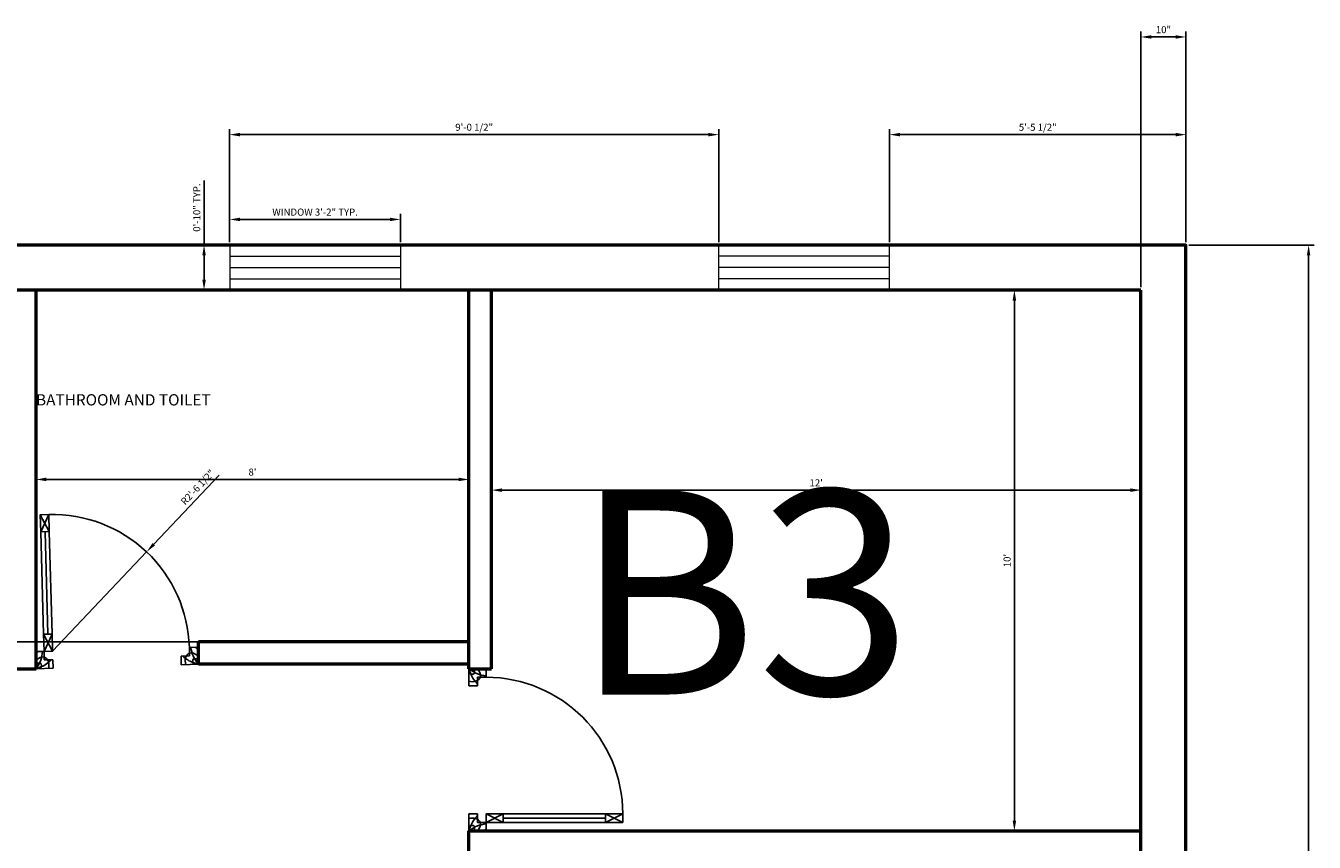
# Model space of a CAD drawing. Units: inches. Extents: x -28 to 484, y -33 to 391.
# Tile 4 of 4: x 199 to 484, y 209 to 391. Entities that reach past the tile are written whole.
import ezdxf

# ---------------------------------------------------------------- set-up
doc = ezdxf.new("R2010")
doc.units = ezdxf.units.IN
for name, color, linetype, lineweight in [('A-ANNO-DIMS', 2, 'Continuous', 18), ('A-AREA-IDEN', 7, 'Continuous', 25), ('A-DOOR', 3, 'Continuous', 25), ('A-GLAZ', 4, 'Continuous', 18), ('A-WALL', 7, 'Continuous', 50)]:
    doc.layers.add(name, color=color, linetype=linetype, lineweight=lineweight)
doc.styles.get("Standard").update_dxf_attribs({"font": 'arial.ttf'})
doc.dimstyles.new('ISO-25', dxfattribs={"dimtxt": 1.5625, "dimasz": 2.3125, "dimexe": 1.25, "dimexo": 0.625, "dimtad": 1, "dimlunit": 4, "dimtxsty": 'Standard', "dimcen": 2.5, "dimadec": 0, "dimazin": 0, "dimtfac": 1, "dimtmove": 0, "dimatfit": 3, "dimfxl": 1, "dimarcsym": 0})

# ---------------------------------------------------------------- blocks, each defined once
blk = doc.blocks.new('A$C05E21637')
for p, q in [((50, 800), (100, 900)), ((100, 800), (50, 900)), ((75, 800), (75, 200)), ((100, 200), (50, 100)), ((50, 200), (100, 100)), ((0, 100), (0, 0)), ((0, 100), (50, 100)), ((50, 100), (50, 50)), ((900, 100), (900, 50)), ((950, 100), (900, 100)), ((950, 100), (950, 0)), ((100, 50), (50, 50)), ((100, 50), (100, 0)), ((850, 50), (900, 50)), ((850, 50), (850, 0)), ((0, 0), (100, 0)), ((950, 0), (850, 0))]:
    blk.add_line(p, q)
for points in [[(50, 800), (100, 800), (100, 900), (50, 900)], [(50, 200), (100, 200), (100, 800), (50, 800)], [(50, 200), (100, 200), (100, 100), (50, 100)]]:
    blk.add_lwpolyline(points, close=True)
blk.add_arc((100, 100), 800, 0, 90)
for points, knots in [([(0, 0), (11.2, 16), (32.5, 46.3), (38.7, 82.7), (41.2, 100)], [0, 0, 0, 0, 57.729567, 109.527977, 109.527977, 109.527977, 109.527977]), ([(950, 0), (938.8, 16), (917.5, 46.3), (911.3, 82.7), (908.8, 100)], [0, 0, 0, 0, 57.729567, 109.527977, 109.527977, 109.527977, 109.527977]), ([(0, 50), (17.5, 61.3), (46.9, 80.3), (79.6, 38.4), (75.6, 13.1), (73.5, 0)], [0, 0, 0, 0, 52.797078, 89.119952, 128.374378, 128.374378, 128.374378, 128.374378]), ([(0, 0), (21.6, 7.2), (55.2, 18.3), (81.2, 41.3), (90.1, 50)], [0, 0, 0, 0, 67.133415, 104.197904, 104.197904, 104.197904, 104.197904]), ([(0, 30.3), (11.9, 32.6), (36.4, 37.4), (31.4, 12.7), (28.8, 0)], [0, 0, 0, 0, 28.773527, 59.024697, 59.024697, 59.024697, 59.024697]), ([(950, 0), (928.4, 7.2), (894.8, 18.3), (868.8, 41.3), (859.9, 50)], [0, 0, 0, 0, 67.133415, 104.197904, 104.197904, 104.197904, 104.197904]), ([(950, 50), (932.5, 61.3), (903.1, 80.3), (870.4, 38.4), (874.4, 13.1), (876.5, 0)], [0, 0, 0, 0, 52.797078, 89.119952, 128.374378, 128.374378, 128.374378, 128.374378]), ([(950, 30.3), (938.1, 32.6), (913.6, 37.4), (918.6, 12.7), (921.2, 0)], [0, 0, 0, 0, 28.773527, 59.024697, 59.024697, 59.024697, 59.024697])]:
    blk.add_open_spline(points, degree=3, knots=knots)
for points in [[(0, 86.7), (4.7, 91.3), (9.4, 95.9), (15.1, 100)], [(950, 86.7), (945.3, 91.3), (940.6, 95.9), (934.9, 100)]]:
    blk.add_open_spline(points, degree=3)
blk = doc.blocks.new('*D4')
at = {"layer": 'A-ANNO-DIMS', "color": 0, "lineweight": -2, "transparency": 16777216}
for p, q in [((416.35, 332), (419.2, 332)), ((417.95, 329.69), (417.95, 214.31)), ((416.35, 212), (419.2, 212))]:
    blk.add_line(p, q, dxfattribs=at)
at = {"layer": 'A-ANNO-DIMS', "color": 0, "transparency": 16777216}
for points in [[(417.56, 329.69), (418.34, 329.69), (417.95, 332)], [(417.56, 214.31), (418.34, 214.31), (417.95, 212)]]:
    blk.add_solid(points, dxfattribs=at)
at = {"layer": 'Defpoints', "color": 0, "transparency": 16777216}
for p in [(415.72, 332), (415.72, 212), (417.95, 212)]:
    blk.add_point(p, dxfattribs=at)
at = {"layer": 'A-ANNO-DIMS', "color": 0, "transparency": 16777216, "insert": (416.53, 272), "char_height": 1.562, "attachment_point": 5, "rotation": 90}
blk.add_mtext("10'", dxfattribs=at)
blk = doc.blocks.new('*D5')
at = {"layer": 'A-ANNO-DIMS', "color": 0, "lineweight": -2, "transparency": 16777216}
for p, q in [((302, 289.38), (302, 286.38)), ((446, 289.38), (446, 286.38)), ((304.31, 287.63), (443.69, 287.63))]:
    blk.add_line(p, q, dxfattribs=at)
at = {"layer": 'A-ANNO-DIMS', "color": 0, "transparency": 16777216}
for points in [[(304.31, 288.01), (304.31, 287.24), (302, 287.63)], [(443.69, 288.01), (443.69, 287.24), (446, 287.63)]]:
    blk.add_solid(points, dxfattribs=at)
at = {"layer": 'Defpoints', "color": 0, "transparency": 16777216}
for p in [(302, 290), (446, 290), (446, 287.63)]:
    blk.add_point(p, dxfattribs=at)
at = {"layer": 'A-ANNO-DIMS', "color": 0, "transparency": 16777216, "insert": (374, 289.04), "char_height": 1.562, "attachment_point": 5}
blk.add_mtext("12'", dxfattribs=at)
blk = doc.blocks.new('*D15')
at = {"layer": 'A-ANNO-DIMS', "color": 0, "lineweight": -2, "transparency": 16777216}
for p, q in [((201, 301.53), (201, 288.75)), ((297, 301.53), (297, 288.75)), ((203.31, 290), (294.69, 290))]:
    blk.add_line(p, q, dxfattribs=at)
at = {"layer": 'A-ANNO-DIMS', "color": 0, "transparency": 16777216}
for points in [[(203.31, 290.39), (203.31, 289.61), (201, 290)], [(294.69, 290.39), (294.69, 289.61), (297, 290)]]:
    blk.add_solid(points, dxfattribs=at)
at = {"layer": 'Defpoints', "color": 0, "transparency": 16777216}
for p in [(201, 302.15), (297, 302.15), (297, 290)]:
    blk.add_point(p, dxfattribs=at)
at = {"layer": 'A-ANNO-DIMS', "color": 0, "transparency": 16777216, "insert": (249, 291.42), "char_height": 1.562, "attachment_point": 5}
blk.add_mtext("8'", dxfattribs=at)
blk = doc.blocks.new('*D16')
at = {"layer": 'A-ANNO-DIMS', "color": 0, "lineweight": -2, "transparency": 16777216}
for p, q in [((456.63, 342), (484.44, 342)), ((483.19, 339.69), (483.19, 2.31)), ((456.63, 0), (484.44, 0))]:
    blk.add_line(p, q, dxfattribs=at)
at = {"layer": 'A-ANNO-DIMS', "color": 0, "transparency": 16777216}
for points in [[(482.8, 339.69), (483.57, 339.69), (483.19, 342)], [(482.8, 2.31), (483.57, 2.31), (483.19, 0)]]:
    blk.add_solid(points, dxfattribs=at)
at = {"layer": 'Defpoints', "color": 0, "transparency": 16777216}
for p in [(456, 342), (456, 0), (483.19, 0)]:
    blk.add_point(p, dxfattribs=at)
at = {"layer": 'A-ANNO-DIMS', "color": 0, "transparency": 16777216, "insert": (481.76, 171), "char_height": 1.562, "attachment_point": 5, "rotation": 90}
blk.add_mtext('28\'-6"', dxfattribs=at)
blk = doc.blocks.new('*D17')
at = {"layer": 'A-ANNO-DIMS', "color": 0, "lineweight": -2, "transparency": 16777216}
for p, q in [((446, 332.63), (446, 389.42)), ((456, 342.62), (456, 389.42)), ((453.69, 388.17), (448.31, 388.17))]:
    blk.add_line(p, q, dxfattribs=at)
at = {"layer": 'A-ANNO-DIMS', "color": 0, "transparency": 16777216}
for points in [[(448.31, 388.56), (448.31, 387.79), (446, 388.17)], [(453.69, 388.56), (453.69, 387.79), (456, 388.17)]]:
    blk.add_solid(points, dxfattribs=at)
at = {"layer": 'Defpoints', "color": 0, "transparency": 16777216}
for p in [(446, 388.17), (456, 342), (446, 332)]:
    blk.add_point(p, dxfattribs=at)
at = {"layer": 'A-ANNO-DIMS', "color": 0, "transparency": 16777216, "insert": (451, 389.59), "char_height": 1.562, "attachment_point": 5}
blk.add_mtext('10"', dxfattribs=at)
blk = doc.blocks.new('WIN-PLAN-FRAME')
for p, q in [((0, 10), (0, 0)), ((37.87, 10), (37.87, 0)), ((0, 7.5), (37.87, 7.5)), ((0, 5), (37.87, 5)), ((0, 2.5), (37.87, 2.5))]:
    blk.add_line(p, q)
blk = doc.blocks.new('*D28')
at = {"layer": 'A-ANNO-DIMS', "color": 0, "lineweight": -2, "transparency": 16777216}
for p, q in [((243.94, 342.62), (243.94, 348.93)), ((281.81, 342.62), (281.81, 348.93)), ((246.26, 347.68), (279.5, 347.68))]:
    blk.add_line(p, q, dxfattribs=at)
at = {"layer": 'A-ANNO-DIMS', "color": 0, "transparency": 16777216}
for points in [[(246.26, 348.07), (246.26, 347.3), (243.94, 347.68)], [(279.5, 348.07), (279.5, 347.3), (281.81, 347.68)]]:
    blk.add_solid(points, dxfattribs=at)
at = {"layer": 'Defpoints', "color": 0, "transparency": 16777216}
for p in [(281.81, 347.68), (243.94, 342), (281.81, 342)]:
    blk.add_point(p, dxfattribs=at)
at = {"layer": 'A-ANNO-DIMS', "color": 0, "transparency": 16777216, "insert": (262.88, 349.11), "char_height": 1.5625, "attachment_point": 5}
blk.add_mtext('WINDOW 3\'-2" TYP.', dxfattribs=at)
blk = doc.blocks.new('*D29')
at = {"layer": 'A-ANNO-DIMS', "color": 0, "lineweight": -2, "transparency": 16777216}
for p, q in [((238.26, 342), (238.26, 356.3)), ((243.32, 342), (237.01, 342)), ((238.26, 334.31), (238.26, 339.69)), ((243.32, 332), (237.01, 332))]:
    blk.add_line(p, q, dxfattribs=at)
at = {"layer": 'A-ANNO-DIMS', "color": 0, "transparency": 16777216}
for points in [[(237.88, 339.69), (238.65, 339.69), (238.26, 342)], [(237.88, 334.31), (238.65, 334.31), (238.26, 332)]]:
    blk.add_solid(points, dxfattribs=at)
at = {"layer": 'Defpoints', "color": 0, "transparency": 16777216}
for p in [(238.26, 342), (243.94, 342), (243.94, 332)]:
    blk.add_point(p, dxfattribs=at)
at = {"layer": 'A-ANNO-DIMS', "color": 0, "transparency": 16777216, "insert": (236.84, 350.31), "char_height": 1.5625, "attachment_point": 5, "rotation": 90}
blk.add_mtext('0\'-10" TYP.', dxfattribs=at)
blk = doc.blocks.new('*D31')
at = {"layer": 'A-ANNO-DIMS', "color": 0, "lineweight": -2, "transparency": 16777216}
for p, q in [((296.38, 332), (-25.8, 332)), ((-24.55, 329.69), (-24.55, 256.31)), ((296.38, 254), (-25.8, 254))]:
    blk.add_line(p, q, dxfattribs=at)
at = {"layer": 'A-ANNO-DIMS', "color": 0, "transparency": 16777216}
for points in [[(-24.93, 329.69), (-24.16, 329.69), (-24.55, 332)], [(-24.93, 256.31), (-24.16, 256.31), (-24.55, 254)]]:
    blk.add_solid(points, dxfattribs=at)
at = {"layer": 'Defpoints', "color": 0, "transparency": 16777216}
for p in [(297, 332), (-24.55, 254), (297, 254)]:
    blk.add_point(p, dxfattribs=at)
at = {"layer": 'A-ANNO-DIMS', "color": 0, "transparency": 16777216, "insert": (-25.97, 293), "char_height": 1.562, "attachment_point": 5, "rotation": 90}
blk.add_mtext('6\'-6"', dxfattribs=at)
blk = doc.blocks.new('*D33')
at = {"layer": 'A-ANNO-DIMS', "color": 0, "lineweight": -2, "transparency": 16777216}
for p, q in [((243.94, 342.62), (243.94, 367.75)), ((246.26, 366.5), (350.07, 366.5)), ((352.38, 342.62), (352.38, 367.75))]:
    blk.add_line(p, q, dxfattribs=at)
at = {"layer": 'A-ANNO-DIMS', "color": 0, "transparency": 16777216}
for points in [[(246.26, 366.89), (246.26, 366.11), (243.94, 366.5)], [(350.07, 366.89), (350.07, 366.11), (352.38, 366.5)]]:
    blk.add_solid(points, dxfattribs=at)
at = {"layer": 'Defpoints', "color": 0, "transparency": 16777216}
for p in [(352.38, 366.5), (243.94, 342), (352.38, 342)]:
    blk.add_point(p, dxfattribs=at)
at = {"layer": 'A-ANNO-DIMS', "color": 0, "transparency": 16777216, "insert": (298.16, 367.93), "char_height": 1.562, "attachment_point": 5}
blk.add_mtext('9\'-0 1/2"', dxfattribs=at)
blk = doc.blocks.new('*D34')
at = {"layer": 'A-ANNO-DIMS', "color": 0, "lineweight": -2, "transparency": 16777216}
for p, q in [((390.25, 342.62), (390.25, 367.75)), ((392.57, 366.5), (453.69, 366.5)), ((456, 342.62), (456, 367.75))]:
    blk.add_line(p, q, dxfattribs=at)
at = {"layer": 'A-ANNO-DIMS', "color": 0, "transparency": 16777216}
for points in [[(392.57, 366.89), (392.57, 366.11), (390.25, 366.5)], [(453.69, 366.89), (453.69, 366.11), (456, 366.5)]]:
    blk.add_solid(points, dxfattribs=at)
at = {"layer": 'Defpoints', "color": 0, "transparency": 16777216}
for p in [(456, 366.5), (390.25, 342), (456, 342)]:
    blk.add_point(p, dxfattribs=at)
at = {"layer": 'A-ANNO-DIMS', "color": 0, "transparency": 16777216, "insert": (423.13, 367.93), "char_height": 1.562, "attachment_point": 5}
blk.add_mtext('5\'-5 1/2"', dxfattribs=at)
blk = doc.blocks.new('*D41')
at = {"layer": 'A-ANNO-DIMS', "color": 0, "lineweight": -2, "transparency": 16777216}
for p, q in [((241.65, 290.97), (227.11, 275.61)), ((204.68, 251.89), (225.52, 273.93))]:
    blk.add_line(p, q, dxfattribs=at)
at = {"layer": 'A-ANNO-DIMS', "color": 0, "transparency": 16777216}
blk.add_solid([(226.83, 275.87), (227.39, 275.34), (225.52, 273.93)], dxfattribs=at)
at = {"layer": 'Defpoints', "color": 0, "transparency": 16777216}
for p in [(225.52, 273.93), (204.68, 251.89)]:
    blk.add_point(p, dxfattribs=at)
at = {"layer": 'A-ANNO-DIMS', "color": 0, "transparency": 16777216, "insert": (236.99, 288.13), "char_height": 1.562, "attachment_point": 5, "rotation": 46.5919}
blk.add_mtext('R2\'-6 1/2"', dxfattribs=at)

msp = doc.modelspace()

# ---------------------------------------------------------------- linework, layer by layer
at = {"layer": 'A-WALL'}
for p, q in [((446, 332), (124, 332)), ((201, 248), (201, 332)), ((297, 248), (297, 332)), ((302, 248), (302, 332)), ((446, 10), (446, 332)), ((297, 254), (237, 254)), ((237, 249), (237, 254)), ((297, 249), (237, 249)), ((196, 248), (201, 248)), ((297, 248), (302, 248)), ((297, 212), (446, 212)), ((297, 207), (297, 212))]:
    msp.add_line(p, q, dxfattribs=at)
msp.add_lwpolyline([(0, 258), (0, 0), (456, 0), (456, 342), (0, 342)], dxfattribs=at)

# ---------------------------------------------------------------- block references
at = {"layer": 'A-DOOR'}
for p, xscale, yscale, zscale, rotation in [((201, 248), 0.0379093539060402, 0.0379093539060402, 0.0379093539060402, 1.591140271195039), ((297, 212), -0.0378947376525429, 0.0378947376525429, 0.0378947376525429, 270)]:
    msp.add_blockref('A$C05E21637', p, dxfattribs=dict(at, xscale=xscale, yscale=yscale, zscale=zscale, rotation=rotation))
at = {"layer": 'A-GLAZ'}
msp.add_blockref('WIN-PLAN-FRAME', (243.943, 332), dxfattribs=at)
at = {"layer": 'A-GLAZ', "rotation": 180}
msp.add_blockref('WIN-PLAN-FRAME', (390.255, 342), dxfattribs=at)

# ---------------------------------------------------------------- texts
at = {"layer": 'A-AREA-IDEN', "attachment_point": 1}
for s, width, insert, char_height in [('BATHROOM AND TOILET', 96, (201, 308.912), 2.5), ('B3', 125.68012, (320.32, 287.626), 45.3593)]:
    msp.add_mtext_dynamic_manual_height_columns(s, width=width, gutter_width=226.796, heights=[0], dxfattribs=dict(at, insert=insert, char_height=char_height))

# ---------------------------------------------------------------- dimensions: what is measured, and where the dimension line sits
at = {"layer": 'A-ANNO-DIMS'}
for base, p1, p2, override, picture, middle in [((446, 388.171), (456, 342), (446, 332), {"dimclrd": 0, "dimclre": 0, "dimclrt": 0}, '*D17', (451, 389.594)), ((352.385, 366.5), (243.943, 342), (352.385, 342), {"dimdec": 1, "dimlfac": 1, "dimrnd": 0, "dimzin": 1, "dimdsep": 46, "dimlunit": 4, "dimfrac": 2}, '*D33', (298.164, 367.933)), ((456, 366.5), (390.255, 342), (456, 342), {"dimdec": 1, "dimlfac": 1, "dimrnd": 0, "dimzin": 1, "dimdsep": 46, "dimlunit": 4, "dimfrac": 2}, '*D34', (423.127, 367.933)), ((297, 290), (201, 302.152), (297, 302.152), {"dimclrd": 0, "dimclre": 0, "dimclrt": 0}, '*D15', (249, 291.423)), ((446, 287.626), (302, 290), (446, 290), {"dimclrd": 0, "dimclre": 0, "dimclrt": 0}, '*D5', (374, 289.036))]:
    dim = msp.add_linear_dim(base=base, p1=p1, p2=p2, dimstyle='ISO-25', override=override, dxfattribs=at)
    dim.commit()
    dim.dimension.update_dxf_attribs({"geometry": picture, "text_midpoint": middle})
dim = msp.add_linear_dim(base=(238.263, 342), p1=(243.943, 332), p2=(243.943, 342), angle=90, text='<> TYP.', dimstyle='ISO-25', override={"dimdec": 1, "dimlfac": 1, "dimrnd": 0, "dimzin": 1, "dimdsep": 46, "dimlunit": 4, "dimfrac": 2}, dxfattribs=at)
dim.commit()
dim.dimension.update_dxf_attribs({"geometry": '*D29', "text_midpoint": (236.84, 350.307)})
dim = msp.add_linear_dim(base=(281.813, 347.681), p1=(243.943, 342), p2=(281.813, 342), text='WINDOW <> TYP.', dimstyle='ISO-25', override={"dimdec": 1, "dimlfac": 1, "dimrnd": 0, "dimzin": 1, "dimdsep": 46, "dimlunit": 4, "dimfrac": 2}, dxfattribs=at)
dim.commit()
dim.dimension.update_dxf_attribs({"geometry": '*D28', "text_midpoint": (262.878, 349.114)})
for base, p1, p2, override, picture, middle in [((483.187, 0), (456, 342), (456, 0), {"dimclrd": 0, "dimclre": 0, "dimclrt": 0}, '*D16', (481.765, 171)), ((-24.546, 254), (297, 332), (297, 254), {"dimdec": 1, "dimlfac": 1, "dimrnd": 0, "dimzin": 1, "dimdsep": 46, "dimlunit": 4, "dimfrac": 2}, '*D31', (-25.969, 293)), ((417.95, 212), (415.724, 332), (415.724, 212), {"dimclrd": 0, "dimclre": 0, "dimclrt": 0}, '*D4', (416.527, 272))]:
    dim = msp.add_linear_dim(base=base, p1=p1, p2=p2, angle=90, dimstyle='ISO-25', override=override, dxfattribs=at)
    dim.commit()
    dim.dimension.update_dxf_attribs({"geometry": picture, "text_midpoint": middle})
dim = msp.add_radius_dim(center=(204.684, 251.895), mpoint=(225.525, 273.927), dimstyle='ISO-25', override={"dimdec": 1, "dimlfac": 1, "dimrnd": 0, "dimzin": 1, "dimdsep": 46, "dimlunit": 4, "dimfrac": 2}, dxfattribs=at)
dim.commit()
dim.dimension.update_dxf_attribs({"geometry": '*D41', "text_midpoint": (238.029, 287.146), "dimtype": 164})

doc.saveas('drawing.dxf')
